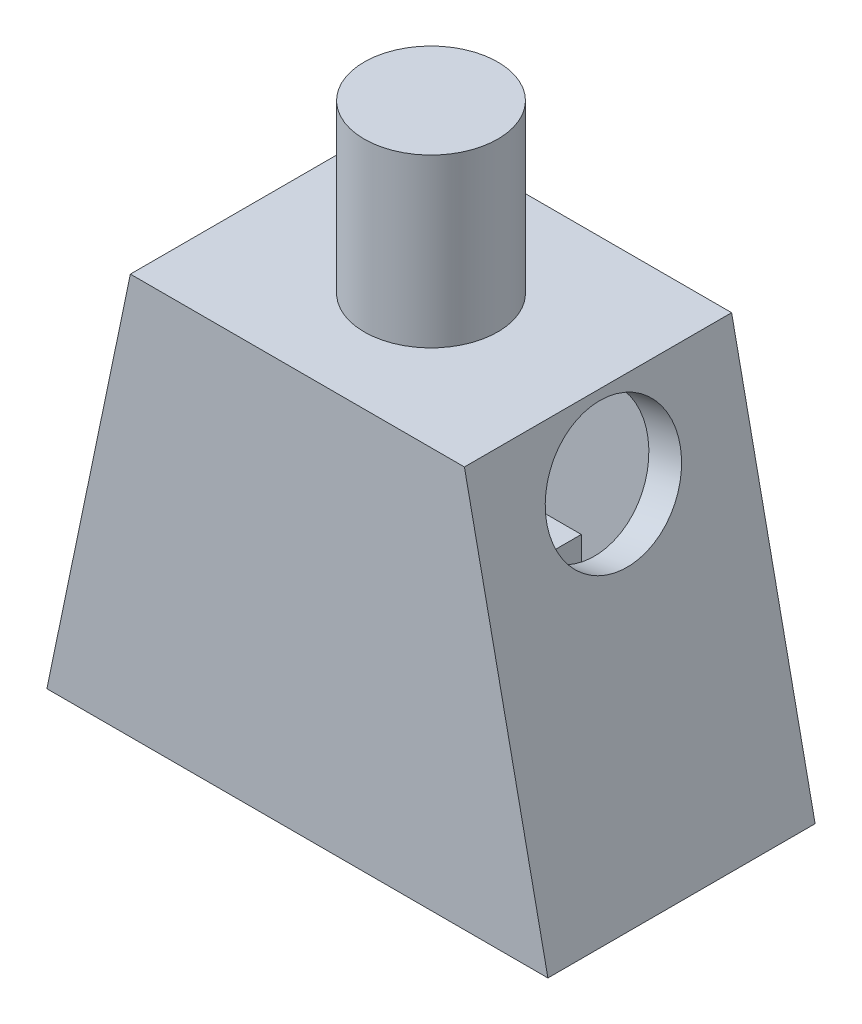
from build123d import *

# Parameters (mm, degrees)
TORSO_BLOCK_DEPTH        = 8
TORSO_SHELL_1MM_T        = -1
NECK_STUD_SKETCH_R       = 2
NECK_STUD_4_DEPTH        = 5
ARM_HOLE_1_3_REACH       = 23.606
ARM_HOLE_1_SKETCH_R      = 2
ARM_HOLE_2_3_REACH       = 26.042
ARM_HOLE_2_SKETCH_R      = 2
HIP_CONNECTOR_SKETCH_W   = 3
HIP_CONNECTOR_SKETCH_H   = 6
HIP_CONNECTOR_BOSS_DEPTH = 5


with BuildPart() as part:
    # Torso Profile Sketch → Torso Block (new body)
    with BuildSketch(Plane.XY):
        Polygon((0, 0), (15, 0), (12.5, 12), (2.5, 12), align=None)
    extrude(amount=-TORSO_BLOCK_DEPTH)

    # Torso Shell 1mm
    torso_shell_1mm_openings = [part.faces().sort_by_distance(p)[0] for p in [
        (7.5, 0, -4),
    ]]
    offset(amount=TORSO_SHELL_1MM_T, openings=torso_shell_1mm_openings, kind=Kind.INTERSECTION)

    # Neck Stud Sketch → Neck Stud Ø4 (add)
    with BuildSketch(Plane(origin=(0, 12, 0), x_dir=(1, 0, 0), z_dir=(0, 1, 0))):
        with Locations(Location((7.5, 4, 0), (0, 0, 270))):
            Circle(NECK_STUD_SKETCH_R)
    extrude(amount=NECK_STUD_4_DEPTH)

    # Arm Hole 1 Sketch → Arm Hole 1 Ø3 (cut, up to next)
    with BuildSketch(Plane(origin=(14.376039933, 2.995008319, 0), x_dir=(0, 0, -1), z_dir=(0.978980419737605, 0.20395425411200113, 0)), mode=Mode.PRIVATE) as arm_hole_1_3_sk1:
        with Locations(Location((4, 6.940686188, 0), (0, 0, 90))):
            Circle(ARM_HOLE_1_SKETCH_R)
    arm_hole_1_3_tool1 = extrude(arm_hole_1_3_sk1.sketch, amount=-ARM_HOLE_1_3_REACH, mode=Mode.PRIVATE) & part.part
    add(arm_hole_1_3_tool1.solids().sort_by_distance((12.960457, 9.789804, -4))[0], mode=Mode.SUBTRACT)

    # Arm Hole 2 Sketch → Arm Hole 2 Ø3 (cut, up to next)
    with BuildSketch(Plane(origin=(0, 0, 0), x_dir=(0, 0, 1), z_dir=(-0.978980419737605, 0.20395425411200113, 0)), mode=Mode.PRIVATE) as arm_hole_2_3_sk1:
        with Locations(Location((-4, 10, 0), (0, 0, 270))):
            Circle(ARM_HOLE_2_SKETCH_R)
    arm_hole_2_3_tool1 = extrude(arm_hole_2_3_sk1.sketch, amount=-ARM_HOLE_2_3_REACH, mode=Mode.PRIVATE) & part.part
    add(arm_hole_2_3_tool1.solids().sort_by_distance((2.039543, 9.789804, -4))[0], mode=Mode.SUBTRACT)

    # Hip Connector Sketch → Hip Connector Boss (add)
    with BuildSketch(Plane.XZ):
        with Locations((7.5, -4)):
            Rectangle(HIP_CONNECTOR_SKETCH_W, HIP_CONNECTOR_SKETCH_H)
    extrude(amount=-HIP_CONNECTOR_BOSS_DEPTH)


solid = part.part
